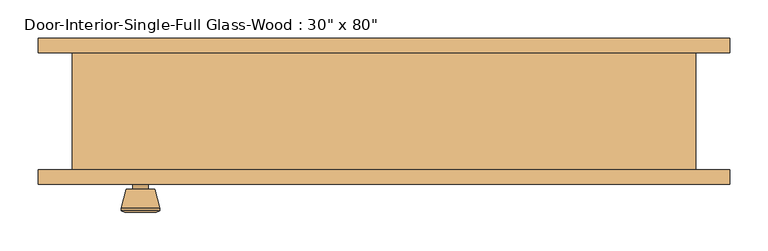
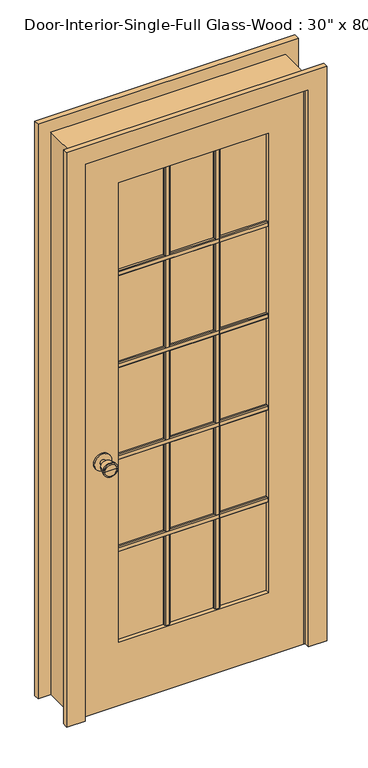
"""IFC4 building model written with IfcOpenShell, lengths in millimetres: door geometry."""

from ifc_helpers import new_model, si_unit, point, frame, frame_2d, origin, place, context, project, spatial, polyline, circle_curve, trimmed, segment, composite_curve, outline, extrude, faceted_brep, source, transform, mapped, element, save
from ifc_brep_helpers import plane_surface, cylinder_surface, revolved_surface, advanced_brep


def door_a0b5ff2a(model_context):
    return source(origin(), model_context, "Body", "SolidModel", [
        extrude(outline(polyline([(-59.055, 1586.23), (-59.055, 1567.18), (-65.405, 1567.18), (-68.58, 1570.355), (-68.58, 1583.055), (-65.405, 1586.23), (-59.055, 1586.23)])), frame((-260.35, 0.0, 0.0), z_axis=(1.0, 0.0, 0.0), x_axis=(0.0, 1.0, 0.0)), (0.0, 0.0, 1.0), 520.7),
        extrude(outline(polyline([(-59.055, 1249.9975), (-59.055, 1230.9475), (-65.405, 1230.9475), (-68.58, 1234.1225), (-68.58, 1246.8225), (-65.405, 1249.9975), (-59.055, 1249.9975)])), frame((-260.35, 0.0, 0.0), z_axis=(1.0, 0.0, 0.0), x_axis=(0.0, 1.0, 0.0)), (0.0, 0.0, 1.0), 520.7),
        extrude(outline(polyline([(-59.055, 913.765), (-59.055, 894.715), (-65.405, 894.715), (-68.58, 897.89), (-68.58, 910.59), (-65.405, 913.765), (-59.055, 913.765)])), frame((-260.35, 0.0, 0.0), z_axis=(1.0, 0.0, 0.0), x_axis=(0.0, 1.0, 0.0)), (0.0, 0.0, 1.0), 520.7),
        extrude(outline(polyline([(-59.055, 577.5325), (-59.055, 558.4825), (-65.405, 558.4825), (-68.58, 561.6575), (-68.58, 574.3575), (-65.405, 577.5325), (-59.055, 577.5325)])), frame((-260.35, 0.0, 0.0), z_axis=(1.0, 0.0, 0.0), x_axis=(0.0, 1.0, 0.0)), (0.0, 0.0, 1.0), 520.7),
        extrude(outline(polyline([(77.2583333, -59.055), (96.3083333, -59.055), (96.3083333, -65.405), (93.1333333, -68.58), (80.4333333, -68.58), (77.2583333, -65.405), (77.2583333, -59.055)])), frame((0.0, 0.0, 231.775), z_axis=(0.0, 0.0, 1.0), x_axis=(1.0, 0.0, 0.0)), (0.0, 0.0, 1.0), 1681.1625),
        extrude(outline(polyline([(-96.3083333, -59.055), (-77.2583333, -59.055), (-77.2583333, -65.405), (-80.4333333, -68.58), (-93.1333333, -68.58), (-96.3083333, -65.405), (-96.3083333, -59.055)])), frame((0.0, 0.0, 231.775), z_axis=(0.0, 0.0, 1.0), x_axis=(1.0, 0.0, 0.0)), (0.0, 0.0, 1.0), 1681.1625),
        extrude(outline(polyline([(-52.07, 1586.23), (-45.72, 1586.23), (-42.545, 1583.055), (-42.545, 1570.355), (-45.72, 1567.18), (-52.07, 1567.18), (-52.07, 1586.23)])), frame((-260.35, 0.0, 0.0), z_axis=(1.0, 0.0, 0.0), x_axis=(0.0, 1.0, 0.0)), (0.0, 0.0, 1.0), 520.7),
        extrude(outline(polyline([(-52.07, 1249.9975), (-45.72, 1249.9975), (-42.545, 1246.8225), (-42.545, 1234.1225), (-45.72, 1230.9475), (-52.07, 1230.9475), (-52.07, 1249.9975)])), frame((-260.35, 0.0, 0.0), z_axis=(1.0, 0.0, 0.0), x_axis=(0.0, 1.0, 0.0)), (0.0, 0.0, 1.0), 520.7),
        extrude(outline(polyline([(-52.07, 913.765), (-45.72, 913.765), (-42.545, 910.59), (-42.545, 897.89), (-45.72, 894.715), (-52.07, 894.715), (-52.07, 913.765)])), frame((-260.35, 0.0, 0.0), z_axis=(1.0, 0.0, 0.0), x_axis=(0.0, 1.0, 0.0)), (0.0, 0.0, 1.0), 520.7),
        extrude(outline(polyline([(-52.07, 577.5325), (-45.72, 577.5325), (-42.545, 574.3575), (-42.545, 561.6575), (-45.72, 558.4825), (-52.07, 558.4825), (-52.07, 577.5325)])), frame((-260.35, 0.0, 0.0), z_axis=(1.0, 0.0, 0.0), x_axis=(0.0, 1.0, 0.0)), (0.0, 0.0, 1.0), 520.7),
        extrude(outline(polyline([(77.2583333, -52.07), (77.2583333, -45.72), (80.4333333, -42.545), (93.1333333, -42.545), (96.3083333, -45.72), (96.3083333, -52.07), (77.2583333, -52.07)])), frame((0.0, 0.0, 231.775), z_axis=(0.0, 0.0, 1.0), x_axis=(1.0, 0.0, 0.0)), (0.0, 0.0, 1.0), 1681.1625),
        extrude(outline(polyline([(-96.3083333, -52.07), (-96.3083333, -45.72), (-93.1333333, -42.545), (-80.4333333, -42.545), (-77.2583333, -45.72), (-77.2583333, -52.07), (-96.3083333, -52.07)])), frame((0.0, 0.0, 231.775), z_axis=(0.0, 0.0, 1.0), x_axis=(1.0, 0.0, 0.0)), (0.0, 0.0, 1.0), 1681.1625),
        advanced_brep(
        [(-317.5, -32.1, 914.4), (-327.5, -32.1, 914.4), (-307.5, -32.1, 914.4), (-297.0241324, 16.9, 914.4), (-337.9758676, 16.9, 914.4), (-317.5, 16.9, 914.4), (-292.5, 15.0721319, 914.4), (-342.5, 15.0721319, 914.4), (-292.5, 11.6084537, 914.4), (-342.5, 11.6084537, 914.4), (-298.863764, -13.1, 914.4), (-336.136236, -13.1, 914.4), (-307.5, -13.1, 914.4), (-327.5, -13.1, 914.4)],
        [
            (0, 1),
            (1, 2, circle_curve(frame((-317.5, -32.1, 914.4), z_axis=(0.0, -1.0, 0.0), x_axis=(-1.0, 0.0, 0.0)), 10.0)),
            (2, 0),
            (2, 1, circle_curve(frame((-317.5, -32.1, 914.4), z_axis=(0.0, -1.0, 0.0), x_axis=(-1.0, 0.0, 0.0)), 10.0)),
            (3, 4, circle_curve(frame((-317.5, 16.9, 914.4), z_axis=(0.0, 1.0, 0.0), x_axis=(-1.0, 0.0, 0.0)), 20.4758676)),
            (4, 5),
            (5, 3),
            (4, 3, circle_curve(frame((-317.5, 16.9, 914.4), z_axis=(0.0, 1.0, 0.0), x_axis=(-1.0, 0.0, 0.0)), 20.4758676)),
            (6, 7, circle_curve(frame((-317.5, 15.0721319, 914.4), z_axis=(0.0, 1.0, 0.0), x_axis=(-1.0, 0.0, 0.0)), 25.0)),
            (7, 4),
            (3, 6),
            (7, 6, circle_curve(frame((-317.5, 15.0721319, 914.4), z_axis=(0.0, 1.0, 0.0), x_axis=(-1.0, 0.0, 0.0)), 25.0)),
            (8, 9, circle_curve(frame((-317.5, 11.6084537, 914.4), z_axis=(0.0, 1.0, 0.0), x_axis=(-1.0, 0.0, 0.0)), 25.0)),
            (9, 7),
            (6, 8),
            (9, 8, circle_curve(frame((-317.5, 11.6084537, 914.4), z_axis=(0.0, 1.0, 0.0), x_axis=(-1.0, 0.0, 0.0)), 25.0)),
            (10, 11, circle_curve(frame((-317.5, -13.1, 914.4), z_axis=(0.0, 1.0, 0.0), x_axis=(-1.0, 0.0, 0.0)), 18.636236)),
            (11, 9),
            (8, 10),
            (11, 10, circle_curve(frame((-317.5, -13.1, 914.4), z_axis=(0.0, 1.0, 0.0), x_axis=(-1.0, 0.0, 0.0)), 18.636236)),
            (12, 13, circle_curve(frame((-317.5, -13.1, 914.4), z_axis=(0.0, 1.0, 0.0), x_axis=(-1.0, 0.0, 0.0)), 10.0)),
            (13, 11),
            (10, 12),
            (13, 12, circle_curve(frame((-317.5, -13.1, 914.4), z_axis=(0.0, 1.0, 0.0), x_axis=(-1.0, 0.0, 0.0)), 10.0)),
            (1, 13),
            (12, 2),
        ],
        [
            plane_surface(frame((-317.5, -32.1, 914.4), z_axis=(0.0, -1.0, 0.0), x_axis=(-1.0, 0.0, 0.0))),
            plane_surface(frame((-317.5, 16.9, 914.4), z_axis=(0.0, 1.0, 0.0), x_axis=(-1.0, 0.0, 0.0))),
            revolved_surface(polyline([(-337.9758676, 16.9, 914.4), (-342.5, 15.0721319, 914.4)]), (-317.5, -32.1, 914.4), (0.0, -1.0, 0.0)),
            cylinder_surface(frame((-317.5, -32.1, 914.4), z_axis=(0.0, -1.0, 0.0), x_axis=(-1.0, 0.0, 0.0)), 25.0),
            revolved_surface(polyline([(-342.5, 11.6084537, 914.4), (-336.136236, -13.1, 914.4)]), (-317.5, -32.1, 914.4), (0.0, -1.0, 0.0)),
            plane_surface(frame((-317.5, -13.1, 914.4), z_axis=(0.0, -1.0, 0.0), x_axis=(-1.0, 0.0, 0.0))),
            cylinder_surface(frame((-317.5, -32.1, 914.4), z_axis=(0.0, -1.0, 0.0), x_axis=(-1.0, 0.0, 0.0)), 10.0),
        ],
        [
            (0, [[1, 2, 3]]),
            (0, [[-3, 4, -1]]),
            (1, [[5, 6, 7]]),
            (1, [[8, -7, -6]]),
            (2, [[9, 10, -5, 11]]),
            (2, [[12, -11, -8, -10]]),
            (3, [[13, 14, -9, 15]]),
            (3, [[16, -15, -12, -14]]),
            (4, [[17, 18, -13, 19]]),
            (4, [[20, -19, -16, -18]]),
            (5, [[21, 22, -17, 23]]),
            (5, [[24, -23, -20, -22]]),
            (6, [[-2, 25, -21, 26]]),
            (6, [[-4, -26, -24, -25]]),
        ],
    ),
        extrude(outline(composite_curve([segment(trimmed(circle_curve(frame_2d((914.4, -317.5)), 30.0), [point((914.4, -347.5))], [point((914.4, -287.5))], False, "CARTESIAN"), True, "CONTINUOUS"), segment(trimmed(circle_curve(frame_2d((914.4, -317.5)), 30.0), [point((914.4, -287.5))], [point((914.4, -347.5))], False, "CARTESIAN"), True, "CONTINUOUS")], self_intersect=False)), frame((0.0, -38.1, 0.0), z_axis=(0.0, 1.0, 0.0), x_axis=(0.0, 0.0, 1.0)), (0.0, 0.0, 1.0), 6.0),
        advanced_brep(
        [(-317.5, -79.025, 914.4), (-307.5, -79.025, 914.4), (-327.5, -79.025, 914.4), (-297.0241324, -128.025, 914.4), (-317.5, -128.025, 914.4), (-337.9758676, -128.025, 914.4), (-292.5, -126.1971319, 914.4), (-342.5, -126.1971319, 914.4), (-292.5, -122.7334537, 914.4), (-342.5, -122.7334537, 914.4), (-298.863764, -98.025, 914.4), (-336.136236, -98.025, 914.4), (-307.5, -98.025, 914.4), (-327.5, -98.025, 914.4)],
        [
            (0, 1),
            (1, 2, circle_curve(frame((-317.5, -79.025, 914.4), z_axis=(0.0, 1.0, 0.0), x_axis=(-1.0, 0.0, 0.0)), 10.0)),
            (2, 0),
            (2, 1, circle_curve(frame((-317.5, -79.025, 914.4), z_axis=(0.0, 1.0, 0.0), x_axis=(-1.0, 0.0, 0.0)), 10.0)),
            (3, 4),
            (4, 5),
            (5, 3, circle_curve(frame((-317.5, -128.025, 914.4), z_axis=(0.0, -1.0, 0.0), x_axis=(-1.0, 0.0, 0.0)), 20.4758676)),
            (3, 5, circle_curve(frame((-317.5, -128.025, 914.4), z_axis=(0.0, -1.0, 0.0), x_axis=(-1.0, 0.0, 0.0)), 20.4758676)),
            (6, 3),
            (5, 7),
            (7, 6, circle_curve(frame((-317.5, -126.1971319, 914.4), z_axis=(0.0, -1.0, 0.0), x_axis=(-1.0, 0.0, 0.0)), 25.0)),
            (6, 7, circle_curve(frame((-317.5, -126.1971319, 914.4), z_axis=(0.0, -1.0, 0.0), x_axis=(-1.0, 0.0, 0.0)), 25.0)),
            (8, 6),
            (7, 9),
            (9, 8, circle_curve(frame((-317.5, -122.7334537, 914.4), z_axis=(0.0, -1.0, 0.0), x_axis=(-1.0, 0.0, 0.0)), 25.0)),
            (8, 9, circle_curve(frame((-317.5, -122.7334537, 914.4), z_axis=(0.0, -1.0, 0.0), x_axis=(-1.0, 0.0, 0.0)), 25.0)),
            (10, 8),
            (9, 11),
            (11, 10, circle_curve(frame((-317.5, -98.025, 914.4), z_axis=(0.0, -1.0, 0.0), x_axis=(-1.0, 0.0, 0.0)), 18.636236)),
            (10, 11, circle_curve(frame((-317.5, -98.025, 914.4), z_axis=(0.0, -1.0, 0.0), x_axis=(-1.0, 0.0, 0.0)), 18.636236)),
            (12, 10),
            (11, 13),
            (13, 12, circle_curve(frame((-317.5, -98.025, 914.4), z_axis=(0.0, -1.0, 0.0), x_axis=(-1.0, 0.0, 0.0)), 10.0)),
            (12, 13, circle_curve(frame((-317.5, -98.025, 914.4), z_axis=(0.0, -1.0, 0.0), x_axis=(-1.0, 0.0, 0.0)), 10.0)),
            (1, 12),
            (13, 2),
        ],
        [
            plane_surface(frame((-317.5, -79.025, 914.4), z_axis=(0.0, 1.0, 0.0), x_axis=(-1.0, 0.0, 0.0))),
            plane_surface(frame((-317.5, -128.025, 914.4), z_axis=(0.0, -1.0, 0.0), x_axis=(-1.0, 0.0, 0.0))),
            revolved_surface(polyline([(-337.9758676, -128.025, 914.4), (-342.5, -126.1971319, 914.4)]), (-317.5, -79.025, 914.4), (0.0, 1.0, 0.0)),
            cylinder_surface(frame((-317.5, -79.025, 914.4), z_axis=(0.0, 1.0, 0.0), x_axis=(-1.0, 0.0, 0.0)), 25.0),
            revolved_surface(polyline([(-342.5, -122.7334537, 914.4), (-336.136236, -98.025, 914.4)]), (-317.5, -79.025, 914.4), (0.0, 1.0, 0.0)),
            plane_surface(frame((-317.5, -98.025, 914.4), z_axis=(0.0, 1.0, 0.0), x_axis=(-1.0, 0.0, 0.0))),
            cylinder_surface(frame((-317.5, -79.025, 914.4), z_axis=(0.0, 1.0, 0.0), x_axis=(-1.0, 0.0, 0.0)), 10.0),
        ],
        [
            (0, [[1, 2, 3]]),
            (0, [[-3, 4, -1]]),
            (1, [[5, 6, 7]]),
            (1, [[-6, -5, 8]]),
            (2, [[9, -7, 10, 11]]),
            (2, [[-10, -8, -9, 12]]),
            (3, [[13, -11, 14, 15]]),
            (3, [[-14, -12, -13, 16]]),
            (4, [[17, -15, 18, 19]]),
            (4, [[-18, -16, -17, 20]]),
            (5, [[21, -19, 22, 23]]),
            (5, [[-22, -20, -21, 24]]),
            (6, [[25, -23, 26, -2]]),
            (6, [[-26, -24, -25, -4]]),
        ],
    ),
        extrude(outline(composite_curve([segment(trimmed(circle_curve(frame_2d((914.4, -317.5)), 30.0), [point((914.4, -347.5))], [point((914.4, -287.5))], False, "CARTESIAN"), True, "CONTINUOUS"), segment(trimmed(circle_curve(frame_2d((914.4, -317.5)), 30.0), [point((914.4, -287.5))], [point((914.4, -347.5))], False, "CARTESIAN"), True, "CONTINUOUS")], self_intersect=False)), frame((0.0, -79.025, 0.0), z_axis=(0.0, 1.0, 0.0), x_axis=(0.0, 0.0, 1.0)), (0.0, 0.0, 1.0), 6.0),
        extrude(outline(polyline([(2032.0, -381.0), (0.0, -381.0), (0.0, 381.0), (2032.0, 381.0), (2032.0, -381.0)]), holes=[polyline([(1912.9375, -260.35), (1912.9375, 260.35), (231.775, 260.35), (231.775, -260.35), (1912.9375, -260.35)])]), frame((0.0, -73.025, 0.0), z_axis=(0.0, 1.0, 0.0), x_axis=(0.0, 0.0, 1.0)), (0.0, 0.0, 1.0), 34.925),
        faceted_brep([(406.4, -73.025, 0.0), (381.0, -73.025, 0.0), (381.0, -38.1, 0.0), (368.3, -38.1, 0.0), (368.3, -3.175, 0.0), (381.0, -3.175, 0.0), (381.0, 79.375, 0.0), (406.4, 79.375, 0.0), (406.4, 79.375, 2057.4), (406.4, -73.025, 2057.4), (381.0, 79.375, 2032.0), (-381.0, 79.375, 2032.0), (-381.0, 79.375, 0.0), (-406.4, 79.375, 0.0), (-406.4, 79.375, 2057.4), (381.0, -3.175, 2032.0), (368.3, -3.175, 2019.3), (-368.3, -3.175, 2019.3), (-368.3, -3.175, 0.0), (-381.0, -3.175, 0.0), (-381.0, -3.175, 2032.0), (368.3, -38.1, 2019.3), (381.0, -38.1, 2032.0), (-381.0, -38.1, 2032.0), (-381.0, -38.1, 0.0), (-368.3, -38.1, 0.0), (-368.3, -38.1, 2019.3), (381.0, -73.025, 2032.0), (-406.4, -73.025, 2057.4), (-406.4, -73.025, 0.0), (-381.0, -73.025, 0.0), (-381.0, -73.025, 2032.0)], [[[0, 1, 2, 3, 4, 5, 6, 7]], [[7, 8, 9, 0]], [[6, 10, 11, 12, 13, 14, 8, 7]], [[5, 15, 10, 6]], [[4, 16, 17, 18, 19, 20, 15, 5]], [[3, 21, 16, 4]], [[2, 22, 23, 24, 25, 26, 21, 3]], [[1, 27, 22, 2]], [[0, 9, 28, 29, 30, 31, 27, 1]], [[8, 14, 28, 9]], [[15, 20, 11, 10]], [[21, 26, 17, 16]], [[27, 31, 23, 22]], [[29, 13, 12, 19, 18, 25, 24, 30]], [[14, 13, 29, 28]], [[20, 19, 12, 11]], [[26, 25, 18, 17]], [[31, 30, 24, 23]]]),
        extrude(outline(polyline([(260.35, -52.07), (260.35, -59.055), (-260.35, -59.055), (-260.35, -52.07), (260.35, -52.07)])), frame((0.0, 0.0, 231.775), z_axis=(0.0, 0.0, 1.0), x_axis=(1.0, 0.0, 0.0)), (0.0, 0.0, 1.0), 1681.1625),
        extrude(outline(polyline([(0.0, 450.85), (2101.85, 450.85), (2101.85, -450.85), (0.0, -450.85), (0.0, -387.35), (2038.35, -387.35), (2038.35, 387.35), (0.0, 387.35), (0.0, 450.85)])), frame((0.0, 79.375, 0.0), z_axis=(0.0, 1.0, 0.0), x_axis=(0.0, 0.0, 1.0)), (0.0, 0.0, 1.0), 19.05),
        extrude(outline(polyline([(0.0, 450.85), (2101.85, 450.85), (2101.85, -450.85), (0.0, -450.85), (0.0, -387.35), (2038.35, -387.35), (2038.35, 387.35), (0.0, 387.35), (0.0, 450.85)])), frame((0.0, -92.075, 0.0), z_axis=(0.0, 1.0, 0.0), x_axis=(0.0, 0.0, 1.0)), (0.0, 0.0, 1.0), 19.05),
    ])


if __name__ == "__main__":
    model = new_model("IFC4")
    model_context = context("Model", 3, world=origin())
    ifc_project = project(units=[si_unit("LENGTHUNIT", "METRE", prefix="MILLI")], contexts=[model_context])
    site = spatial("IfcSite", under=ifc_project)
    building = spatial("IfcBuilding", under=site)
    placement = place(None, origin())
    door_shape = door_a0b5ff2a(model_context)
    element("IfcDoor", 1, ObjectType="Door-Interior-Single-Full Glass-Wood : 30\" x 80\"", at=placement, inside=building, context=model_context, shape_type="MappedRepresentation", body=[
        mapped(door_shape, transform((0.0, 0.0, 0.0), x_axis=(1.0, 0.0, 0.0), y_axis=(0.0, 1.0, 0.0), z_axis=(0.0, 0.0, 1.0))),
    ])
    save(model, "model.ifc")

# Revit data of these elements
# Type "Door-Interior-Single-Full Glass-Wood : 30\" x 80\""
#   Type Mark = "10"
#   Assembly Code = "C1020300"
#   Analytic Construction = "Wood frame with single clear glass"
#   Top Rail = 0' - 4 11/16"
#   Thickness = 0' - 1 3/8"
#   Thermal Resistance (R) = 1.0102 (h·ft²·°F)/BTU
#   Swing Angle [instance default] = 90.00°
#   Stiles = 0' - 4 3/4"
#   Rough Width = 2' - 8"
#   Rough Height = 6' - 9"
#   Height = 6' - 8"
#   Width = 2' - 6"
#   Heat Transfer Coefficient (U) = 0.9900 BTU/(h·ft²·°F)
#   Bottom Rail = 0' - 9 1/8"
#   Show Grill [instance default] = yes
#   Trim Material = Cherry
#   Panel Material = Cherry
#   Frame Material = Cherry
#   Door Handle Material = Aluminum
#   Visual Light Transmittance = 0
#   Solar Heat Gain Coefficient = 0
#   Wall Closure = (empty or 0)
#   Function = (empty or 0)
# Element 1 (IfcDoor, "Door-Interior-Single-Full Glass-Wood : 30\" x 80\"")
#   Materials on its faces: "Cherry", "Aluminum", "Glass"
# Materials
#   "Cherry": class "Wood", colour RGB 226 177 128, transparency 0, Description = "Prunus Serotina", Cost = 0
#   "Aluminum": class "Metal", colour RGB 247 247 247, transparency 0, Description = "Aluminum 6061", Cost = 0
#   "Glass": class "Glass", colour RGB 0 128 192, transparency 0.75, Description = "Soda Lime Glass", Cost = 0
